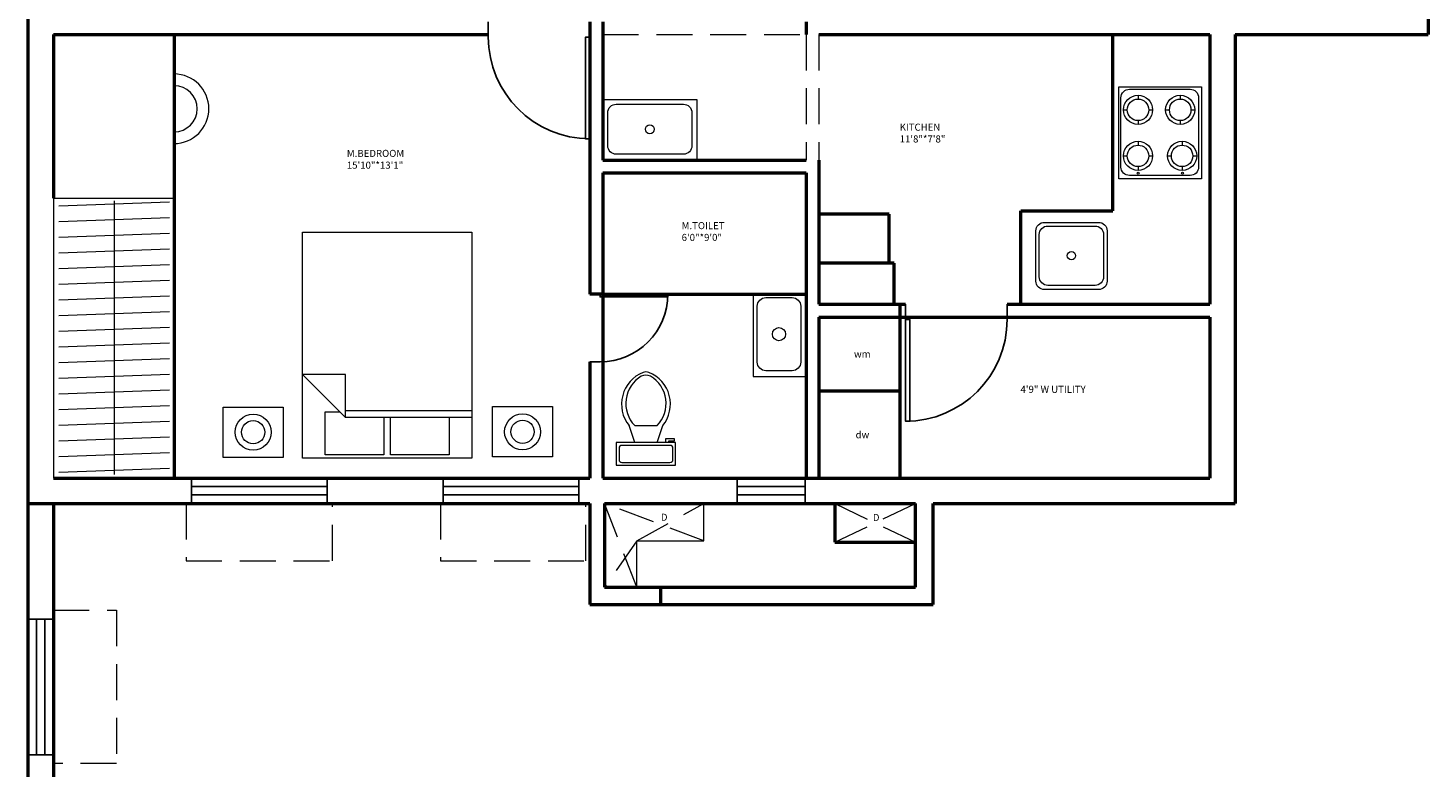
# Model space of a CAD drawing. Units: inches. Extents: x 4795 to 6024, y 2716 to 5025.
# Tile 17 of 19: x 5528 to 6024, y 4414 to 4676. Entities that reach past the tile are written whole.
import ezdxf

# ---------------------------------------------------------------- set-up
doc = ezdxf.new("R2010")
doc.units = ezdxf.units.IN
doc.linetypes.add('DASHED', pattern=[19.05, 12.7, -6.35])
for name, color, linetype, lineweight in [('A-ANNO-TEXT', 7, 'Continuous', 18), ('A-AREA-IDEN', 3, 'Continuous', 18), ('A-DOOR', 4, 'Continuous', 25), ('A-FLOR-FIXT', 9, 'Continuous', 18), ('A-FURN', 8, 'Continuous', 18), ('A-GLAZ', 4, 'Continuous', 25), ('A-WALL', 7, 'Continuous', 50), ('A-WALL-OVHD', 8, 'DASHED', 18)]:
    doc.layers.add(name, color=color, linetype=linetype, lineweight=lineweight)
doc.styles.get("Standard").update_dxf_attribs({"font": 'arial.ttf'})

# ---------------------------------------------------------------- blocks, each defined once
blk = doc.blocks.new('*U2')
for p, q in [((0, 0), (0, -6)), ((40, 0), (40, -6))]:
    blk.add_line(p, q)
blk.add_lwpolyline([(0, 0), (0, 40), (1.75, 40), (1.75, 0)], close=True)
blk.add_arc((0, 0), 40, 0, 90)
blk = doc.blocks.new('Bed - Queen')
for p, q in [((0, -80.00003), (0, 0)), ((0, 0), (59.99999, 0)), ((59.99999, 0), (59.99999, -80.00003)), ((7.99999, -1.2), (28.79998, -1.2)), ((7.99999, -14.4), (7.99999, -1.2)), ((28.79998, -1.2), (28.79998, -14.4)), ((31.19999, -1.2), (51.99999, -1.2)), ((31.19999, -14.4), (31.19999, -1.2)), ((51.99999, -1.2), (51.99999, -16.4)), ((0, -14.4), (44.8, -14.4)), ((59.99999, -29.6), (44.8, -14.4)), ((44.8, -14.4), (44.8, -29.6)), ((44.8, -16.8), (0, -16.8)), ((51.99999, -16.4), (46.79936, -16.4)), ((44.8, -29.6), (59.99999, -29.6)), ((59.99999, -80.00003), (0, -80.00003))]:
    blk.add_line(p, q)
blk = doc.blocks.new('Toilet - top')
for p, q in [((9.5, -6), (9.5, -2)), ((-10, -8.5), (-8, -8.5)), ((-10, -9.5), (-10, -8.5)), ((-7, -9.5), (-10, -9.5)), ((-8, -8.5), (-8, -8)), ((-7, -8), (-7, -9.5)), ((-4, -8), (-6, -14)), ((4, -8), (6, -14)), ((4, -14), (-4, -14))]:
    blk.add_line(p, q)
blk.add_lwpolyline([(10.5, -8), (10.5, 0), (-10.5, 0), (-10.5, -8)], close=True)
for points in [[(-9.5, -2), (-9.5, -6)], [(8.5, -1), (-8.5, -1)], [(-8.5, -7), (8.5, -7)]]:
    blk.add_lwpolyline(points)
for centre, radius, start, end in [((-8.62, -1.88), 0.884, 81.8699, 188.1301), ((8.62, -1.88), 0.884, 351.8699, 98.1301), ((-8.62, -6.12), 0.884, 171.8699, 278.1301), ((8.62, -6.12), 0.884, 261.8699, 8.1301), ((3.52, -21.58), 12.17, 141.4691, 247.9714), ((4.2, -21.82), 11.33, 136.3677, 238.9468), ((-3.52, -21.58), 12.17, 292.0284, 38.5307), ((-4.2, -21.82), 11.33, 301.053, 43.6321), ((0, -27.88), 4, 245.7318, 294.2682), ((0, -29), 4, 254.8605, 285.1395)]:
    blk.add_arc(centre, radius, start, end)
blk = doc.blocks.new('WIN-48')
for p, q in [((0, 0), (0, 48)), ((0, 48), (9, 48)), ((3, 0), (3, 48)), ((6, 48), (6, 0)), ((9, 48), (9, 0)), ((9, 0), (0, 0))]:
    blk.add_line(p, q)
blk = doc.blocks.new('WIN-24')
for p, q in [((0, 0), (0, 9)), ((0, 9), (24, 9)), ((0, 6), (24, 6)), ((24, 9), (24, 0)), ((24, 3), (0, 3)), ((24, 0), (0, 0))]:
    blk.add_line(p, q)
blk = doc.blocks.new('COOKTOP-4B')
for p, q in [((6.77, 29.57), (6.77, 28.22)), ((21.7, 29.57), (21.7, 28.22)), ((1.61, 24.41), (2.97, 24.41)), ((6.77, 20.61), (6.77, 19.25)), ((10.57, 24.41), (11.93, 24.41)), ((16.54, 24.41), (17.9, 24.41)), ((21.7, 20.61), (21.7, 19.25)), ((25.51, 24.41), (26.87, 24.41)), ((6.77, 13.27), (6.77, 11.91)), ((22.37, 13.27), (22.37, 11.91)), ((1.61, 8.11), (2.97, 8.11)), ((10.57, 8.11), (11.93, 8.11)), ((17.2, 8.11), (18.56, 8.11)), ((26.17, 8.11), (27.53, 8.11)), ((6.77, 4.3), (6.77, 2.94)), ((22.37, 4.3), (22.37, 2.94))]:
    blk.add_line(p, q)
blk.add_lwpolyline([(0, 32.52), (29.24, 32.52), (29.24, 0), (0, 0)], close=True)
blk.add_lwpolyline([(3.72, 31.71), (25.19, 31.71, -0.414214), (28.19, 28.71), (28.19, 4.17, -0.414214), (25.19, 1.17), (3.72, 1.17, -0.414214), (0.72, 4.17), (0.72, 28.71, -0.414214)], format="xyb", close=True)
for centre, radius in [((6.77, 24.41), 5.16), ((6.77, 24.41), 3.8), ((21.7, 24.41), 5.16), ((21.7, 24.41), 3.8), ((6.77, 8.11), 5.16), ((6.77, 8.11), 3.8), ((22.37, 8.11), 5.16), ((22.37, 8.11), 3.8), ((6.77, 2), 0.353), ((22.47, 2), 0.353)]:
    blk.add_circle(centre, radius)

msp = doc.modelspace()

# ---------------------------------------------------------------- linework, layer by layer
at = {"layer": 'A-FLOR-FIXT'}
msp.add_lwpolyline([(5731.72, 4629.48), (5765.13, 4629.48), (5765.13, 4650.82), (5731.72, 4650.82)], close=True, dxfattribs=at)
for points in [[(5736.52, 4649.31), (5760.3, 4649.31, -0.414214), (5763.3, 4646.31), (5763.3, 4634.6, -0.414214), (5760.3, 4631.6), (5736.52, 4631.6, -0.414214), (5733.52, 4634.6), (5733.52, 4646.31, -0.414214)], [(5888.11, 4607.49), (5907.32, 4607.49, -0.414214), (5910.32, 4604.49), (5910.32, 4586.7, -0.414214), (5907.32, 4583.7), (5888.11, 4583.7, -0.414214), (5885.11, 4586.7), (5885.11, 4604.49, -0.414214)], [(5889.31, 4606.19), (5906.05, 4606.19, -0.414214), (5909.05, 4603.19), (5909.05, 4588.17, -0.414214), (5906.05, 4585.17), (5889.31, 4585.17, -0.414214), (5886.31, 4588.17), (5886.31, 4603.19, -0.414214)]]:
    msp.add_lwpolyline(points, format="xyb", close=True, dxfattribs=at)
for centre, radius in [((5748.41, 4640.45), 1.59), ((5897.68, 4595.68), 1.48)]:
    msp.add_circle(centre, radius, dxfattribs=at)
at = {"layer": 'A-FURN'}
for p, q in [((5537.22, 4616.09), (5537.22, 4516.98)), ((5537.22, 4616.09), (5579.95, 4616.09)), ((5539.17, 4613.31), (5578.38, 4614.7)), ((5558.78, 4615.05), (5558.78, 4518.2)), ((5539.17, 4607.77), (5578.38, 4609.16)), ((5539.17, 4602.23), (5578.38, 4603.62)), ((5539.17, 4596.69), (5578.38, 4598.07)), ((5539.17, 4591.15), (5578.38, 4592.53)), ((5539.17, 4585.6), (5578.38, 4586.99)), ((5539.17, 4580.06), (5578.38, 4581.45)), ((5539.17, 4574.52), (5578.38, 4575.91)), ((5539.17, 4568.98), (5578.38, 4570.37)), ((5539.17, 4563.44), (5578.38, 4564.83)), ((5539.17, 4557.9), (5578.38, 4559.29)), ((5539.17, 4552.36), (5578.38, 4553.74)), ((5539.17, 4546.81), (5578.38, 4548.2)), ((5539.17, 4541.27), (5578.38, 4542.66)), ((5539.17, 4535.73), (5578.38, 4537.12)), ((5539.17, 4530.19), (5578.38, 4531.58)), ((5539.17, 4524.65), (5578.38, 4526.04)), ((5539.17, 4519.11), (5578.38, 4520.5)), ((5767.47, 4494.73), (5767.47, 4507.98)), ((5743.77, 4478.32), (5743.77, 4494.73)), ((5743.77, 4494.73), (5767.47, 4494.73))]:
    msp.add_line(p, q, dxfattribs=at)
for points in [[(5803.72, 4582.12), (5784.98, 4582.12), (5784.98, 4552.96), (5803.72, 4552.96)], [(5597.31, 4542.12), (5618.58, 4542.12), (5618.58, 4524.29), (5597.31, 4524.29)], [(5692.71, 4542.28), (5713.98, 4542.28), (5713.98, 4524.45), (5692.71, 4524.45)]]:
    msp.add_lwpolyline(points, close=True, dxfattribs=at)
msp.add_lwpolyline([(5789.46, 4580.83), (5798.82, 4580.83, -0.414214), (5801.82, 4577.83), (5801.82, 4557.98, -0.414214), (5798.82, 4554.98), (5789.46, 4554.98, -0.414214), (5786.46, 4557.98), (5786.46, 4577.83, -0.414214)], format="xyb", close=True, dxfattribs=at)
for centre, radius in [((5794.14, 4567.91), 2.32), ((5607.95, 4533.2), 6.37), ((5607.95, 4533.2), 4.11), ((5703.35, 4533.36), 6.37), ((5703.35, 4533.36), 4.11)]:
    msp.add_circle(centre, radius, dxfattribs=at)
for radius in [12.31, 8.17]:
    msp.add_arc((5579.95, 4647.69), radius, 270, 90, dxfattribs=at)
at = {"layer": 'A-WALL'}
for p, q in [((6023.95, 4820.98), (6023.95, 4673.98)), ((5528.22, 4754.09), (5528.22, 4616.09)), ((5727.22, 4678.48), (5727.22, 4582.12)), ((5731.72, 4678.48), (5731.72, 4629.48)), ((5803.72, 4678.48), (5803.72, 4673.98)), ((5537.22, 4673.98), (5691.22, 4673.98)), ((5537.22, 4673.98), (5537.22, 4616.09)), ((5579.95, 4674.06), (5579.95, 4516.98)), ((5808.22, 4673.98), (5946.72, 4673.98)), ((5912.35, 4611.6), (5912.35, 4673.98)), ((5946.72, 4673.98), (5946.72, 4578.48)), ((5955.72, 4673.98), (5955.72, 4507.98)), ((5955.72, 4673.98), (6023.95, 4673.98)), ((5731.72, 4629.48), (5803.72, 4629.48)), ((5808.22, 4629.48), (5808.22, 4578.48)), ((5731.72, 4624.98), (5803.72, 4624.98)), ((5731.72, 4624.98), (5731.72, 4516.98)), ((5803.72, 4624.98), (5803.72, 4516.98)), ((5528.22, 4616.09), (5528.22, 4507.98)), ((5833.11, 4610.33), (5808.22, 4610.33)), ((5833.11, 4593.03), (5833.11, 4610.33)), ((5879.72, 4578.48), (5879.72, 4611.6)), ((5879.72, 4611.6), (5912.35, 4611.6)), ((5834.87, 4593.03), (5808.22, 4593.03)), ((5834.87, 4578.48), (5834.87, 4593.03)), ((5731.72, 4582.12), (5727.22, 4582.12)), ((5731.72, 4582.12), (5803.72, 4582.12)), ((5808.22, 4578.48), (5838.94, 4578.48)), ((5836.9, 4578.48), (5836.9, 4516.98)), ((5874.94, 4578.48), (5946.72, 4578.48)), ((5808.22, 4573.98), (5946.72, 4573.98)), ((5808.22, 4573.98), (5808.22, 4516.98)), ((5946.72, 4573.98), (5946.72, 4516.98)), ((5727.22, 4558.12), (5727.22, 4516.98)), ((5836.9, 4547.73), (5808.22, 4547.73)), ((5537.22, 4516.98), (5727.22, 4516.98)), ((5731.72, 4516.98), (5946.72, 4516.98)), ((5528.22, 4507.98), (5727.22, 4507.98)), ((5528.22, 4507.98), (5528.22, 3920.81)), ((5537.22, 4507.98), (5537.22, 4368.81)), ((5727.22, 4507.98), (5727.22, 4472.2)), ((5732.37, 4507.98), (5732.37, 4478.32)), ((5732.37, 4507.98), (5842.45, 4507.98)), ((5813.89, 4507.98), (5813.89, 4494.23)), ((5842.45, 4478.32), (5842.45, 4507.98)), ((5848.78, 4472.2), (5848.78, 4507.98)), ((5848.78, 4507.98), (5955.72, 4507.98)), ((5813.89, 4494.23), (5842.45, 4494.23)), ((5732.37, 4478.32), (5842.45, 4478.32)), ((5752.15, 4478.32), (5752.15, 4472.2)), ((5727.22, 4472.2), (5848.78, 4472.2))]:
    msp.add_line(p, q, dxfattribs=at)
at = {"layer": 'A-WALL-OVHD'}
for p, q in [((5731.72, 4673.98), (5803.72, 4673.98)), ((5803.72, 4673.98), (5803.72, 4629.48)), ((5808.22, 4673.98), (5808.22, 4629.48)), ((5584.19, 4507.98), (5584.19, 4487.71)), ((5636.03, 4487.71), (5636.03, 4507.98)), ((5674.28, 4507.98), (5674.28, 4487.71)), ((5725.73, 4487.71), (5725.73, 4507.98)), ((5767.47, 4494.73), (5732.37, 4507.98)), ((5743.77, 4478.32), (5732.37, 4507.98)), ((5743.77, 4494.73), (5767.47, 4507.98)), ((5813.89, 4507.98), (5842.45, 4494.23)), ((5813.89, 4494.23), (5842.45, 4507.98)), ((5743.77, 4494.73), (5732.37, 4478.32)), ((5584.19, 4487.71), (5636.03, 4487.71)), ((5674.28, 4487.71), (5725.73, 4487.71)), ((5537.22, 4470.16), (5559.56, 4470.16)), ((5559.56, 4470.16), (5559.56, 4415.95)), ((5559.56, 4415.95), (5537.22, 4415.95))]:
    msp.add_line(p, q, dxfattribs=at)

# ---------------------------------------------------------------- block references
at = {"layer": 'A-DOOR'}
for p, xscale, yscale, zscale, rotation in [((5727.22, 4673.08), 0.9, 0.9, 0.9, 180), ((5730.82, 4582.12), 0.6, 0.6, 0.6, 270), ((5838.94, 4573.08), -0.9, 0.9, 0.9, 180)]:
    msp.add_blockref('*U2', p, dxfattribs=dict(at, xscale=xscale, yscale=yscale, zscale=zscale, rotation=rotation))
at = {"layer": 'A-FLOR-FIXT'}
msp.add_blockref('COOKTOP-4B', (5914.51, 4622.9), dxfattribs=at)
at = {"layer": 'A-FLOR-FIXT', "rotation": 180}
msp.add_blockref('Toilet - top', (5747.04, 4521.53), dxfattribs=at)
at = {"layer": 'A-FURN', "rotation": 180}
msp.add_blockref('Bed - Queen', (5685.41, 4524.05), dxfattribs=at)
at = {"layer": 'A-GLAZ'}
for name, p, rotation in [('WIN-48', (5586.11, 4516.98), 269.9999999999991), ('WIN-48', (5675.28, 4516.98), 269.9999999999987), ('WIN-24', (5803.36, 4516.98), 180), ('WIN-48', (5537.22, 4467.06), 180)]:
    msp.add_blockref(name, p, dxfattribs=dict(at, rotation=rotation))

# ---------------------------------------------------------------- texts
at = {"layer": 'A-ANNO-TEXT', "char_height": 2.5, "attachment_point": 1}
for s, width, insert in [('wm', 16.9449, (5820.69, 4562.13)), ('dw', 12.0008, (5821.26, 4533.55)), ('D', 3.1704, (5752.32, 4504.36)), ('D', 3.1742, (5827.38, 4504.29))]:
    msp.add_mtext_dynamic_manual_height_columns(s, width=width, gutter_width=12.5, heights=[0], dxfattribs=dict(at, insert=insert))
at = {"layer": 'A-AREA-IDEN', "char_height": 2.5, "attachment_point": 1}
for s, width, insert in [('KITCHEN\\P11\'8"*7\'8"', 50.9806, (5836.88, 4642.42)), ('M.BEDROOM\\P15\'10"*13\'1"', 70.0022, (5641.12, 4633.15)), ('M.TOILET\\P6\'0"*9\'0"', 47.5849, (5759.67, 4607.57)), ('4\'9" W UTILITY', 54.1092, (5879.65, 4549.63))]:
    msp.add_mtext_dynamic_manual_height_columns(s, width=width, gutter_width=12.5, heights=[0], dxfattribs=dict(at, insert=insert))

doc.saveas('drawing.dxf')
